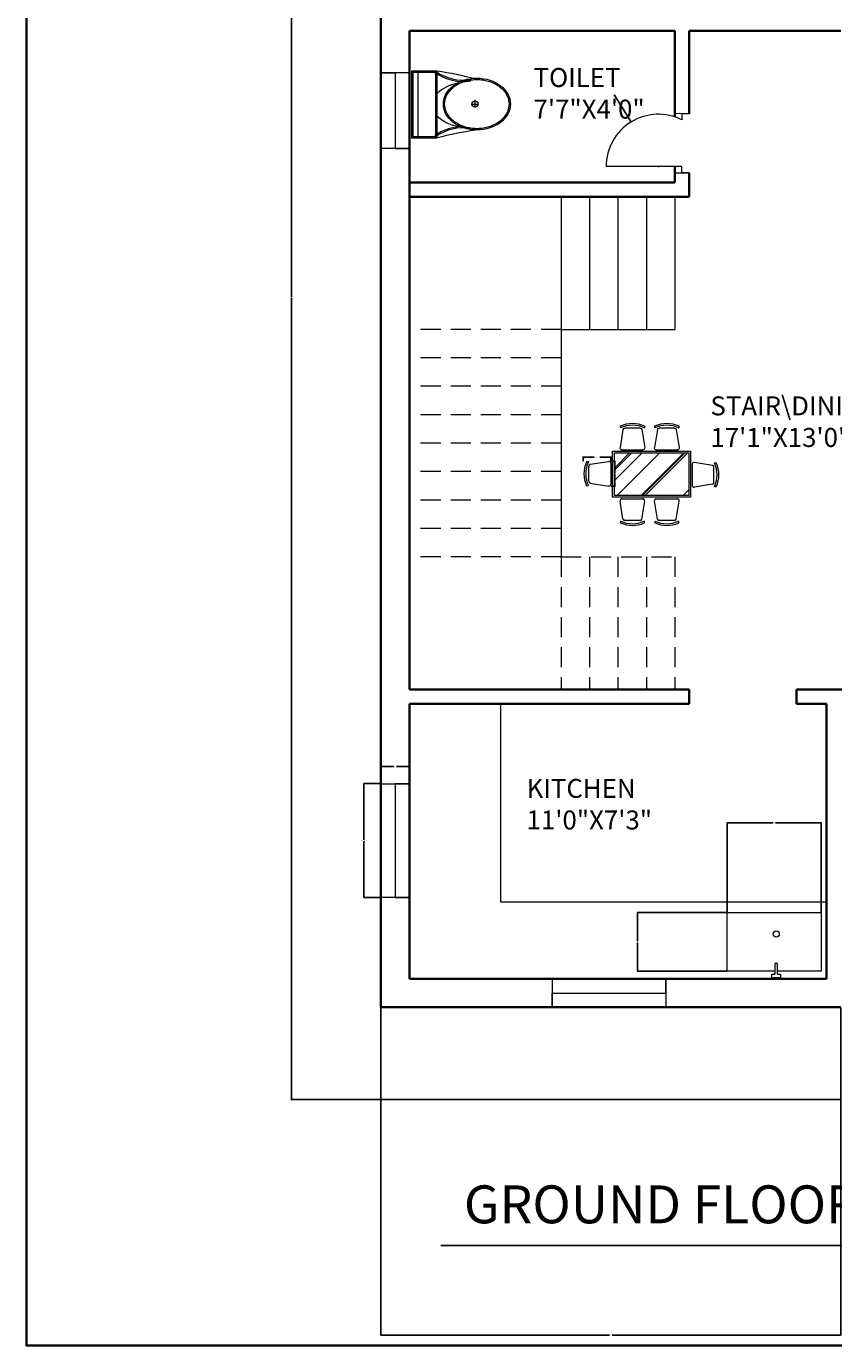
# Model space of a CAD drawing. Units: inches. Extents: x 1832 to 2989, y 1644 to 2902.
# Tile 1 of 8: x 1832 to 2087, y 1644 to 2061. Entities that reach past the tile are written whole.
import ezdxf

# ---------------------------------------------------------------- set-up
doc = ezdxf.new("R2010")
doc.units = ezdxf.units.IN
doc.linetypes.add('DASHED2', pattern=[9.525, 6.35, -3.175])
for name, color, linetype, lineweight in [('A-ANNO-DIMS', 2, 'Continuous', 18), ('A-ANNO-TEXT', 7, 'Continuous', 25), ('A-ANNO-TTLB', 7, 'Continuous', 35), ('A-AREA-IDEN', 7, 'Continuous', 18), ('A-DOOR', 3, 'Continuous', 18), ('A-FLOR-CASE', 8, 'Continuous', 18), ('A-FLOR-FIXT', 9, 'Continuous', 18), ('A-FLOR-STRS', 7, 'Continuous', 18), ('A-FLOR-STRS-OVHD', 254, 'DASHED2', 13), ('A-FURN', 8, 'Continuous', 18), ('A-FURN-PATT', 252, 'Continuous', 13), ('A-GLAZ', 4, 'Continuous', 18), ('A-WALL', 7, 'Continuous', 35)]:
    doc.layers.add(name, color=color, linetype=linetype, lineweight=lineweight)
doc.styles.get("Standard").update_dxf_attribs({"font": 'arial.ttf'})
doc.dimstyles.get("Standard").update_dxf_attribs({"dimtxt": 0.18, "dimasz": 0.18, "dimexe": 0.18, "dimexo": 0.0625, "dimgap": 0.09, "dimtad": 0, "dimtih": 1, "dimtoh": 1, "dimdec": 4, "dimzin": 0, "dimdsep": 46, "dimtxsty": 'Standard', "dimcen": 0.09, "dimadec": 0, "dimazin": 0, "dimtfac": 1, "dimtdec": 4, "dimtofl": 0, "dimtmove": 0, "dimatfit": 3, "dimfxl": 1, "dimtolj": 1, "dimtzin": 0, "dimarcsym": 0})

# ---------------------------------------------------------------- blocks, each defined once
blk = doc.blocks.new('A$C31115884')
for p, q in [((258, 466), (258, 523)), ((283, 498), (223, 498)), ((0, 200), (0, 0)), ((520, 200), (0, 200)), ((10, 190), (10, 10)), ((510, 190), (10, 190)), ((510, 10), (510, 190)), ((520, 0), (520, 200)), ((510, 54), (0, 54)), ((10, 10), (510, 10)), ((0, 0), (520, 0))]:
    blk.add_line(p, q)
blk.add_circle((256, 496), 23.6)
for centre, radius, start, end in [((2778, -205), 2807, 165.4549, 171.7133), ((-295, 403), 365, 324.2091, 9.3499), ((-295, 403), 375, 324.2091, 9.3499), ((139, 406), 293, 315.8436, 2.6563), ((806, 403), 365, 170.6501, 215.7909), ((3237, 905), 2807, 188.2867, 194.5451), ((384, 406), 293, 190.2774, 224.1564), ((806, 403), 375, 179.2036, 215.7909)]:
    blk.add_arc(centre, radius, start, end)
blk.add_ellipse((256, 510), major_axis=(0, -261), ratio=0.772727)
blk.add_open_spline([(256, 259), (263, 259), (270, 260), (288, 262), (299, 265), (320, 273), (330, 278), (350, 291), (360, 299), (378, 316), (386, 326), (402, 347), (409, 358), (421, 383), (427, 395), (436, 422), (440, 436), (445, 465), (447, 480), (448, 509), (448, 524), (445, 553), (443, 568), (436, 596), (432, 610), (422, 636), (416, 649), (402, 672), (395, 683), (379, 703), (370, 712), (351, 728), (341, 735), (321, 746), (310, 751), (289, 757), (278, 759), (256, 761), (245, 761), (223, 757), (212, 754), (191, 746), (181, 741), (161, 728), (151, 720), (133, 703), (125, 693), (110, 672), (103, 660), (90, 636), (85, 623), (76, 596), (72, 582), (67, 553), (66, 538), (64, 509), (65, 494), (68, 465), (70, 450), (77, 422), (81, 408), (91, 382), (97, 370), (111, 346), (118, 335), (135, 316), (144, 307), (162, 291), (172, 284), (193, 273), (203, 269), (225, 262), (236, 260), (250, 259), (253, 259), (256, 259)], degree=3, knots=[0, 0, 0, 0, 0.110105, 0.110105, 0.285049, 0.285049, 0.459994, 0.459994, 0.634938, 0.634938, 0.809882, 0.809882, 0.984827, 0.984827, 1.159771, 1.159771, 1.334715, 1.334715, 1.50966, 1.50966, 1.684604, 1.684604, 1.859549, 1.859549, 2.034493, 2.034493, 2.209437, 2.209437, 2.384382, 2.384382, 2.559326, 2.559326, 2.73427, 2.73427, 2.909215, 2.909215, 3.084159, 3.084159, 3.259103, 3.259103, 3.434048, 3.434048, 3.608992, 3.608992, 3.783936, 3.783936, 3.958881, 3.958881, 4.133825, 4.133825, 4.30877, 4.30877, 4.483714, 4.483714, 4.658658, 4.658658, 4.833603, 4.833603, 5.008547, 5.008547, 5.183491, 5.183491, 5.358436, 5.358436, 5.53338, 5.53338, 5.708324, 5.708324, 5.883269, 5.883269, 6.058213, 6.058213, 6.233158, 6.233158, 6.283185, 6.283185, 6.283185, 6.283185])
blk = doc.blocks.new('CHAIR-DINING')
for p, q in [((0.57, 8.47), (7.25, 8.47)), ((0.93, 2.02), (0, 7.73)), ((6.9, 2.02), (7.83, 7.73)), ((0.12, 1.4), (0.14, 0.86)), ((6.32, 1.56), (1.51, 1.56)), ((7.71, 0.84), (7.69, 1.42))]:
    blk.add_line(p, q)
for centre, radius, start, end in [((0.57, 7.92), 0.547, 90, 192.3792), ((7.25, 7.92), 0.547, 346.3053, 90), ((3.9, 9.34), 8.78, 244.6873, 295.6189), ((3.95, 8.89), 8.89, 244.649, 295.0455), ((1.51, 2.11), 0.547, 193.6947, 269.5544), ((6.32, 2.11), 0.547, 270.4456, 346.3053)]:
    blk.add_arc(centre, radius, start, end)
blk = doc.blocks.new('WIN-PLAN-24IN')
for p, q in [((0, 9), (0, 0)), ((24, 4.5), (24, 9)), ((24, 9), (24, 0)), ((0, 0), (0, 4.5)), ((0, 4.5), (24, 4.5))]:
    blk.add_line(p, q)
blk = doc.blocks.new('WIN-PLAN-36IN')
for p, q in [((0, 9), (0, 0)), ((36, 4.5), (36, 9)), ((36, 9), (36, 0)), ((0, 0), (0, 4.5)), ((0, 4.5), (36, 4.5))]:
    blk.add_line(p, q)
blk = doc.blocks.new('WIN-PLAN-36IN-2')
for p, q in [((0, 36), (9, 36)), ((9, 36), (4.5, 36)), ((4.5, 36), (4.5, 0)), ((9, 0), (0, 0)), ((4.5, 0), (9, 0))]:
    blk.add_line(p, q)
blk = doc.blocks.new('DOOR-PLAN-WC')
for p, q in [((21.75, 18.87), (26.25, 18.72)), ((26.25, 18.72), (24, 18.8)), ((24, 18.8), (24, 16.8)), ((24, 2), (0, 2)), ((21.75, 0), (26.25, 0)), ((24, 0), (24, 2)), ((26.25, 0), (24, 0))]:
    blk.add_line(p, q)
blk.add_arc((16.56, 2), 16.56, 63.308, 180)
blk = doc.blocks.new('*D29')
at = {"layer": 'A-ANNO-DIMS', "color": 0, "lineweight": -2, "transparency": 16777216}
for p, q in [((2007.84, 1923.49), (2007.84, 1924.92)), ((2008.02, 1924.74), (2011.33, 1924.74)), ((2016.41, 1924.74), (2013.1, 1924.74)), ((2016.59, 1923.49), (2016.59, 1924.92))]:
    blk.add_line(p, q, dxfattribs=at)
at = {"layer": 'A-ANNO-DIMS', "color": 0, "transparency": 16777216}
for points in [[(2008.02, 1924.77), (2008.02, 1924.71), (2007.84, 1924.74)], [(2016.41, 1924.77), (2016.41, 1924.71), (2016.59, 1924.74)]]:
    blk.add_solid(points, dxfattribs=at)
at = {"layer": 'Defpoints', "color": 0, "transparency": 16777216}
for p in [(2016.59, 1924.74), (2007.84, 1923.42), (2016.59, 1923.42)]:
    blk.add_point(p, dxfattribs=at)
at = {"layer": 'A-ANNO-DIMS', "color": 0, "transparency": 16777216, "insert": (2012.21, 1924.74), "char_height": 0.18, "attachment_point": 5}
blk.add_mtext('\\A1;CHAIR 9 TYP.', dxfattribs=at)
blk = doc.blocks.new('*D30')
at = {"layer": 'A-ANNO-DIMS', "color": 0, "lineweight": -2, "transparency": 16777216}
for p, q in [((2016.65, 1923.42), (2018.08, 1923.42)), ((2017.9, 1923.24), (2017.9, 1919.69)), ((2017.9, 1915.78), (2017.9, 1919.33)), ((2016.65, 1915.6), (2018.08, 1915.6))]:
    blk.add_line(p, q, dxfattribs=at)
at = {"layer": 'A-ANNO-DIMS', "color": 0, "transparency": 16777216}
for points in [[(2017.87, 1923.24), (2017.93, 1923.24), (2017.9, 1923.42)], [(2017.87, 1915.78), (2017.93, 1915.78), (2017.9, 1915.6)]]:
    blk.add_solid(points, dxfattribs=at)
at = {"layer": 'Defpoints', "color": 0, "transparency": 16777216}
for p in [(2016.59, 1923.42), (2016.59, 1915.6), (2017.9, 1915.6)]:
    blk.add_point(p, dxfattribs=at)
at = {"layer": 'A-ANNO-DIMS', "color": 0, "transparency": 16777216, "insert": (2017.9, 1919.51), "char_height": 0.18, "attachment_point": 5}
blk.add_mtext('\\A1;8 TYP.', dxfattribs=at)
blk = doc.blocks.new('*D57')
at = {"layer": 'A-ANNO-DIMS', "color": 0, "lineweight": -2, "transparency": 16777216}
for p, q in [((1943.83, 1821.42), (1938.31, 1821.42)), ((1938.49, 1821.24), (1938.49, 1803.6)), ((1938.49, 1785.6), (1938.49, 1803.23)), ((1943.83, 1785.42), (1938.31, 1785.42))]:
    blk.add_line(p, q, dxfattribs=at)
at = {"layer": 'A-ANNO-DIMS', "color": 0, "transparency": 16777216}
for points in [[(1938.46, 1821.24), (1938.52, 1821.24), (1938.49, 1821.42)], [(1938.46, 1785.6), (1938.52, 1785.6), (1938.49, 1785.42)]]:
    blk.add_solid(points, dxfattribs=at)
at = {"layer": 'Defpoints', "color": 0, "transparency": 16777216}
for p in [(1938.49, 1821.42), (1943.89, 1821.42), (1943.89, 1785.42)]:
    blk.add_point(p, dxfattribs=at)
at = {"layer": 'A-ANNO-DIMS', "color": 0, "transparency": 16777216, "insert": (1938.49, 1803.42), "char_height": 0.18, "attachment_point": 5}
blk.add_mtext('\\A1;WINDOW 36 TYP.', dxfattribs=at)
blk = doc.blocks.new('*D58')
at = {"layer": 'A-ANNO-DIMS', "color": 0, "lineweight": -2, "transparency": 16777216}
for p, q in [((1943.89, 1821.48), (1943.89, 1827)), ((1944.07, 1826.82), (1947.93, 1826.82)), ((1952.71, 1826.82), (1948.85, 1826.82)), ((1952.89, 1821.48), (1952.89, 1827))]:
    blk.add_line(p, q, dxfattribs=at)
at = {"layer": 'A-ANNO-DIMS', "color": 0, "transparency": 16777216}
for points in [[(1944.07, 1826.85), (1944.07, 1826.79), (1943.89, 1826.82)], [(1952.71, 1826.85), (1952.71, 1826.79), (1952.89, 1826.82)]]:
    blk.add_solid(points, dxfattribs=at)
at = {"layer": 'Defpoints', "color": 0, "transparency": 16777216}
for p in [(1952.89, 1826.82), (1943.89, 1821.42), (1952.89, 1821.42)]:
    blk.add_point(p, dxfattribs=at)
at = {"layer": 'A-ANNO-DIMS', "color": 0, "transparency": 16777216, "insert": (1948.39, 1826.82), "char_height": 0.18, "attachment_point": 5}
blk.add_mtext('\\A1;9 TYP.', dxfattribs=at)
blk = doc.blocks.new('*D72')
at = {"layer": 'A-ANNO-DIMS', "color": 0, "lineweight": -2, "transparency": 16777216}
for p, q in [((1943.83, 2229.17), (1915.41, 2229.17)), ((1915.59, 2228.99), (1915.59, 1975.53)), ((1915.59, 1721.7), (1915.59, 1975.17)), ((2089.33, 1721.52), (1915.41, 1721.52))]:
    blk.add_line(p, q, dxfattribs=at)
at = {"layer": 'A-ANNO-DIMS', "color": 0, "transparency": 16777216}
for points in [[(1915.56, 2228.99), (1915.62, 2228.99), (1915.59, 2229.17)], [(1915.56, 1721.7), (1915.62, 1721.7), (1915.59, 1721.52)]]:
    blk.add_solid(points, dxfattribs=at)
at = {"layer": 'Defpoints', "color": 0, "transparency": 16777216}
for p in [(1915.59, 2229.17), (1943.89, 2229.17), (2089.39, 1721.52)]:
    blk.add_point(p, dxfattribs=at)
at = {"layer": 'A-ANNO-DIMS', "color": 0, "transparency": 16777216, "insert": (1915.59, 1975.35), "char_height": 0.18, "attachment_point": 5}
blk.add_mtext('\\A1;507.6', dxfattribs=at)
blk = doc.blocks.new('*D75')
at = {"layer": 'A-ANNO-DIMS', "color": 0, "lineweight": -2, "transparency": 16777216}
for p, q in [((1943.89, 1750.61), (1943.89, 1646.75)), ((2089.39, 1750.61), (2089.39, 1646.75)), ((1944.07, 1646.93), (2016.25, 1646.93)), ((2089.21, 1646.93), (2017.03, 1646.93))]:
    blk.add_line(p, q, dxfattribs=at)
at = {"layer": 'A-ANNO-DIMS', "color": 0, "transparency": 16777216}
for points in [[(1944.07, 1646.96), (1944.07, 1646.9), (1943.89, 1646.93)], [(2089.21, 1646.96), (2089.21, 1646.9), (2089.39, 1646.93)]]:
    blk.add_solid(points, dxfattribs=at)
at = {"layer": 'Defpoints', "color": 0, "transparency": 16777216}
for p in [(1943.89, 1750.67), (2089.39, 1750.67), (2089.39, 1646.93)]:
    blk.add_point(p, dxfattribs=at)
at = {"layer": 'A-ANNO-DIMS', "color": 0, "transparency": 16777216, "insert": (2016.64, 1646.93), "char_height": 0.18, "attachment_point": 5}
blk.add_mtext('\\A1;145.5', dxfattribs=at)
blk = doc.blocks.new('*D79')
at = {"layer": 'A-ANNO-DIMS', "color": 0, "lineweight": -2, "transparency": 16777216}
for p, q in [((2053.41, 1780.75), (2053.41, 1809.16)), ((2053.59, 1808.98), (2067.86, 1808.98)), ((2083.06, 1808.98), (2068.79, 1808.98)), ((2083.24, 1780.75), (2083.24, 1809.16))]:
    blk.add_line(p, q, dxfattribs=at)
at = {"layer": 'A-ANNO-DIMS', "color": 0, "transparency": 16777216}
for points in [[(2053.59, 1809.01), (2053.59, 1808.95), (2053.41, 1808.98)], [(2083.06, 1809.01), (2083.06, 1808.95), (2083.24, 1808.98)]]:
    blk.add_solid(points, dxfattribs=at)
at = {"layer": 'Defpoints', "color": 0, "transparency": 16777216}
for p in [(2083.24, 1808.98), (2053.41, 1780.68), (2083.24, 1780.68)]:
    blk.add_point(p, dxfattribs=at)
at = {"layer": 'A-ANNO-DIMS', "color": 0, "transparency": 16777216, "insert": (2068.33, 1808.98), "char_height": 0.18, "attachment_point": 5}
blk.add_mtext('\\A1;29.833', dxfattribs=at)
blk = doc.blocks.new('*D80')
at = {"layer": 'A-ANNO-DIMS', "color": 0, "lineweight": -2, "transparency": 16777216}
for p, q in [((2053.35, 1780.68), (2024.93, 1780.68)), ((2025.11, 1780.5), (2025.11, 1771.56)), ((2025.11, 1762.26), (2025.11, 1771.2)), ((2053.35, 1762.08), (2024.93, 1762.08))]:
    blk.add_line(p, q, dxfattribs=at)
at = {"layer": 'A-ANNO-DIMS', "color": 0, "transparency": 16777216}
for points in [[(2025.08, 1780.5), (2025.14, 1780.5), (2025.11, 1780.68)], [(2025.08, 1762.26), (2025.14, 1762.26), (2025.11, 1762.08)]]:
    blk.add_solid(points, dxfattribs=at)
at = {"layer": 'Defpoints', "color": 0, "transparency": 16777216}
for p in [(2025.11, 1780.68), (2053.41, 1780.68), (2053.41, 1762.08)]:
    blk.add_point(p, dxfattribs=at)
at = {"layer": 'A-ANNO-DIMS', "color": 0, "transparency": 16777216, "insert": (2025.11, 1771.38), "char_height": 0.18, "attachment_point": 5}
blk.add_mtext('\\A1;18.61', dxfattribs=at)
blk = doc.blocks.new('*D127')
at = {"layer": 'A-ANNO-DIMS', "color": 0, "lineweight": -2, "transparency": 16777216}
for p, q in [((2017.62, 2039.25), (2017.8, 2039.25)), ((2017.8, 2039.25), (2022.92, 2030.95)), ((2031.61, 2016.7), (2031.79, 2016.7)), ((2031.7, 2016.61), (2031.7, 2016.79))]:
    blk.add_line(p, q, dxfattribs=at)
at = {"layer": 'A-ANNO-DIMS', "color": 0, "transparency": 16777216}
blk.add_solid([(2022.94, 2030.96), (2022.89, 2030.93), (2023.01, 2030.8)], dxfattribs=at)
at = {"layer": 'Defpoints', "color": 0, "transparency": 16777216}
for p in [(2023.01, 2030.8), (2031.7, 2016.7)]:
    blk.add_point(p, dxfattribs=at)
at = {"layer": 'A-ANNO-DIMS', "color": 0, "transparency": 16777216, "insert": (2017.14, 2039.25), "char_height": 0.18, "attachment_point": 5}
blk.add_mtext('\\A1;R16.56', dxfattribs=at)

msp = doc.modelspace()

# ---------------------------------------------------------------- hatches: boundary and pattern name
at = {"layer": 'A-FURN-PATT'}
h = msp.add_hatch(dxfattribs=at)
h.set_pattern_fill('AR-RROOF', color=256, scale=0.368444, angle=45, style=0)
h.set_pattern_definition([(45, (1517.465, 2118.481), (7.94093, 21.1758), [140.3771, -18.717, 46.7924, -9.3585]), (45, (1522.958, 2130.591), (-15.41863, 2.18375), [28.0754, -3.0883, 56.1508, -7.01885]), (45, (1515.149, 2127.4145), (29.977, 38.84437), [74.8678, -13.10186, 37.4339, -9.3585])])
h.paths.add_polyline_path([(2017.7478, 1926.1046), (2017.7478, 1912.603), (2041.3439, 1912.603), (2041.3439, 1926.1046)])

# ---------------------------------------------------------------- linework, layer by layer
at = {"layer": 'A-ANNO-TEXT'}
msp.add_line((1962.8459, 1675.2337), (2280.5653, 1675.2337), dxfattribs=at)
at = {"layer": 'A-ANNO-TTLB'}
msp.add_lwpolyline([(1831.6677, 2901.9044), (2988.9144, 2901.9044), (2988.9144, 1643.5851), (1831.6677, 1643.5851)], close=True, dxfattribs=at)
at = {"layer": 'A-FLOR-CASE'}
for p, q in [((1981.754, 1846.6726), (1981.754, 1784.0547)), ((1981.754, 1784.0547), (2084.8904, 1784.0547))]:
    msp.add_line(p, q, dxfattribs=at)
at = {"layer": 'A-FLOR-FIXT'}
for points in [[(2068.5195, 1762.076), (2053.4086, 1762.076), (2053.4086, 1780.6849), (2083.2418, 1780.6849), (2083.2418, 1762.076), (2069.3589, 1762.076)], [(2069.3589, 1761.1417), (2069.3589, 1764.4617), (2068.5195, 1764.4617), (2068.5195, 1761.1417)], [(2069.3589, 1761.1417), (2070.335, 1761.1417), (2070.335, 1759.9628), (2067.6253, 1759.9628), (2067.6253, 1761.1417), (2068.5195, 1761.1417)]]:
    msp.add_lwpolyline(points, dxfattribs=at)
msp.add_circle((2068.9811, 1773.831), 0.9741, dxfattribs=at)
at = {"layer": 'A-FLOR-STRS'}
for p, q in [((1952.8904, 2007.1726), (2000.8904, 2007.1726)), ((2000.8904, 2007.1726), (2000.8904, 1959.1726)), ((2000.8904, 2007.1726), (2000.8904, 1965.1726)), ((2009.8904, 2007.1726), (2009.8904, 1965.1726)), ((2018.8904, 2007.1726), (2018.8904, 1965.1726)), ((2027.8904, 2007.1726), (2027.8904, 1965.1726)), ((2036.8904, 2007.1726), (2036.8904, 1965.1726)), ((2000.8904, 1965.1726), (2036.8904, 1965.1726)), ((2000.8904, 1959.1726), (2000.8904, 1893.1726))]:
    msp.add_line(p, q, dxfattribs=at)
at = {"layer": 'A-FLOR-STRS-OVHD'}
for p, q in [((2000.8904, 1965.1726), (1952.8904, 1965.1726)), ((2000.8904, 1956.1726), (1952.8904, 1956.1726)), ((2000.8904, 1947.1726), (1952.8904, 1947.1726)), ((2000.8904, 1938.1726), (1952.8904, 1938.1726)), ((2000.8904, 1929.1726), (1952.8904, 1929.1726)), ((2000.8904, 1920.1726), (1952.8904, 1920.1726)), ((2000.8904, 1911.1726), (1952.8904, 1911.1726)), ((2000.8904, 1902.1726), (1952.8904, 1902.1726)), ((2000.8904, 1893.1726), (1952.8904, 1893.1726)), ((2000.8904, 1893.1726), (2000.8904, 1851.1726)), ((2000.8904, 1893.1726), (2036.8904, 1893.1726)), ((2009.8904, 1893.1726), (2009.8904, 1851.1726)), ((2018.8904, 1893.1726), (2018.8904, 1851.1726)), ((2027.8904, 1893.1726), (2027.8904, 1851.1726)), ((2036.8904, 1893.1726), (2036.8904, 1851.1726))]:
    msp.add_line(p, q, dxfattribs=at)
at = {"layer": 'A-FURN'}
for p, q in [((2042.359, 1922.4877), (2042.359, 1915.8087)), ((2048.803, 1922.1324), (2043.0983, 1923.0614)), ((2049.2644, 1916.7417), (2049.2644, 1921.5547)), ((2049.4269, 1922.9372), (2049.9717, 1922.9171)), ((2048.803, 1916.1639), (2043.0983, 1915.2349)), ((2049.9918, 1915.3468), (2049.4067, 1915.367))]:
    msp.add_line(p, q, dxfattribs=at)
for points in [[(2017.1952, 1926.6572), (2041.8965, 1926.6572), (2041.8965, 1912.0503), (2017.1952, 1912.0503)], [(2017.7478, 1926.1046), (2041.3439, 1926.1046), (2041.3439, 1912.603), (2017.7478, 1912.603)]]:
    msp.add_lwpolyline(points, close=True, dxfattribs=at)
for centre, radius, start, end in [((2042.9062, 1922.4877), 0.5471, 77.620777, 180), ((2048.7173, 1921.5504), 0.5471, 0.445647, 76.305274), ((2041.4901, 1919.1632), 8.7797, 334.381056, 25.312705), ((2041.9373, 1919.1105), 8.8905, 334.954464, 25.350959), ((2048.6266, 1916.7779), 0.6388, 286.031111, 356.752573), ((2042.9787, 1915.8439), 0.6206, 183.254478, 281.116612)]:
    msp.add_arc(centre, radius, start, end, dxfattribs=at)
at = {"layer": 'A-WALL'}
for p, q in [((1943.8904, 2229.1726), (1943.8904, 1750.6726)), ((1943.8904, 2229.1726), (1943.8904, 1750.6726)), ((1943.8904, 2229.1726), (1943.8904, 1750.6726)), ((1952.8904, 2059.6726), (2036.8904, 2059.6726)), ((1952.8904, 2059.6726), (1952.8904, 1851.1726)), ((2036.8904, 2059.6726), (2036.8904, 2032.4253)), ((2041.3904, 2059.6726), (2041.3904, 2033.4226)), ((2041.3904, 2059.6726), (2089.3904, 2059.6726)), ((2036.8904, 2016.6983), (2036.8904, 2011.6726)), ((2041.3904, 2014.6983), (2041.3904, 2007.1726)), ((1952.8904, 2011.6726), (2036.8904, 2011.6726)), ((1952.8904, 2007.1726), (2041.3904, 2007.1726)), ((1952.8904, 1851.1726), (2010.6177, 1851.1726)), ((2010.6177, 1851.1726), (2041.3904, 1851.1726)), ((2041.3904, 1851.1726), (2041.3904, 1846.6726)), ((2075.4242, 1851.1726), (2075.4242, 1846.6726)), ((2075.4242, 1851.1726), (2096.7965, 1851.1726)), ((1952.8904, 1846.6726), (2010.6177, 1846.6726)), ((1952.8904, 1846.6726), (1952.8904, 1759.6726)), ((2041.3904, 1846.6726), (2010.6177, 1846.6726)), ((2041.3904, 1849.0845), (2041.3904, 1846.6726)), ((2075.4242, 1846.6726), (2084.8904, 1846.6726)), ((2084.8904, 1846.6726), (2084.8904, 1759.6726)), ((1952.8904, 1759.6726), (2084.8904, 1759.6726)), ((1952.8904, 1750.6726), (1943.8904, 1750.6726)), ((1952.8904, 1750.6726), (2089.3904, 1750.6726))]:
    msp.add_line(p, q, dxfattribs=at)

# ---------------------------------------------------------------- block references
at = {"layer": 'A-DOOR'}
msp.add_blockref('DOOR-PLAN-WC', (2015.1404, 2014.6983), dxfattribs=at)
at = {"layer": 'A-FLOR-FIXT', "xscale": 0.0406268506401408, "yscale": 0.0406268506401408, "zscale": 0.0406268506401408, "rotation": 269.9999999999998}
msp.add_blockref('A$C31115884', (1953.5142, 2046.8898), dxfattribs=at)
at = {"layer": 'A-FURN', "extrusion": (0, 0, -1), "zscale": -1, "rotation": 180}
for p in [(-2019.5519, 1935.4903), (-2030.4428, 1935.4903)]:
    msp.add_blockref('CHAIR-DINING', p, dxfattribs=at)
at = {"layer": 'A-FURN', "rotation": 269.9999999432575}
msp.add_blockref('CHAIR-DINING', (2008.1214, 1923.4234), dxfattribs=at)
at = {"layer": 'A-FURN'}
for p in [(2019.5519, 1903.1223), (2030.4428, 1903.1223)]:
    msp.add_blockref('CHAIR-DINING', p, dxfattribs=at)
at = {"layer": 'A-GLAZ', "rotation": 270.0000000000013}
msp.add_blockref('WIN-PLAN-24IN', (1943.8904, 2046.3857), dxfattribs=at)
at = {"layer": 'A-GLAZ'}
for name, p in [('WIN-PLAN-36IN-2', (1943.8904, 1785.4153)), ('WIN-PLAN-36IN', (1998.0413, 1750.6726))]:
    msp.add_blockref(name, p, dxfattribs=at)

# ---------------------------------------------------------------- texts
at = {"layer": 'A-ANNO-TEXT', "insert": (1970.1351, 1694.2857), "char_height": 12, "attachment_point": 1}
msp.add_mtext_dynamic_manual_height_columns('GROUND FLOOR EAST FACING PLAN', width=528.005294, gutter_width=12.5, heights=[0], dxfattribs=at)
at = {"layer": 'A-AREA-IDEN', "char_height": 6, "attachment_point": 1}
for s, width, insert in [('TOILET\\P7\'7"X4\'0"', 102.121913, (1992.1671, 2047.8855)), ('STAIR\\\\DINING\\P17\'1"X13\'0"', 222.625783, (2048.147, 1943.978)), ('KITCHEN\\P11\'0"X7\'3"', 205.6642, (1989.9623, 1822.9307))]:
    msp.add_mtext_dynamic_manual_height_columns(s, width=width, gutter_width=12.5, heights=[0], dxfattribs=dict(at, insert=insert))

# ---------------------------------------------------------------- dimensions: what is measured, and where the dimension line sits
at = {"layer": 'A-ANNO-DIMS'}
for base, p1, p2, override, picture, middle in [((1915.5904, 2229.1726), (2089.3904, 1721.5243), (1943.8904, 2229.1726), {"dimdec": 1, "dimlfac": 1, "dimrnd": 0, "dimzin": 0, "dimdsep": 46, "dimlunit": 2}, '*D72', (1915.5904, 1975.3484)), ((2025.1086, 1780.6849), (2053.4086, 1762.076), (2053.4086, 1780.6849), {"dimdec": 2, "dimlfac": 1, "dimrnd": 0, "dimzin": 0, "dimdsep": 46, "dimlunit": 2}, '*D80', (2025.1086, 1771.3805))]:
    dim = msp.add_linear_dim(base=base, p1=p1, p2=p2, angle=90, dimstyle='Standard', override=override, dxfattribs=at)
    dim.commit()
    dim.dimension.update_dxf_attribs({"geometry": picture, "text_midpoint": middle})
dim = msp.add_radius_dim(center=(2031.7013, 2016.6983), mpoint=(2023.0103, 2030.7955), dimstyle='Standard', override={"dimdec": 2, "dimlfac": 1, "dimrnd": 0, "dimzin": 0, "dimdsep": 46, "dimlunit": 2}, dxfattribs=at)
dim.commit()
dim.dimension.update_dxf_attribs({"geometry": '*D127', "text_midpoint": (2017.1359, 2039.2538), "dimtype": 164})
for base, p1, p2, angle, text, picture, middle in [((2016.5901, 1924.7366), (2007.8357, 1923.4234), (2016.5901, 1923.4234), 360, 'CHAIR <> TYP.', '*D29', (2012.2129, 1924.7366)), ((2017.9033, 1915.597), (2016.5901, 1923.4234), (2016.5901, 1915.597), 270, '<> TYP.', '*D30', (2017.9033, 1919.5102)), ((1938.4904, 1821.4153), (1943.8904, 1785.4153), (1943.8904, 1821.4153), 90, 'WINDOW <> TYP.', '*D57', (1938.4904, 1803.4153))]:
    dim = msp.add_linear_dim(base=base, p1=p1, p2=p2, angle=angle, text=text, dimstyle='Standard', override={"dimdec": 0, "dimlfac": 1, "dimrnd": 0, "dimzin": 0, "dimdsep": 46, "dimlunit": 2}, dxfattribs=at)
    dim.commit()
    dim.dimension.update_dxf_attribs({"geometry": picture, "text_midpoint": middle})
dim = msp.add_linear_dim(base=(1952.8904, 1826.8153), p1=(1943.8904, 1821.4153), p2=(1952.8904, 1821.4153), text='<> TYP.', dimstyle='Standard', override={"dimdec": 0, "dimlfac": 1, "dimrnd": 0, "dimzin": 0, "dimdsep": 46, "dimlunit": 2}, dxfattribs=at)
dim.commit()
dim.dimension.update_dxf_attribs({"geometry": '*D58', "text_midpoint": (1948.3904, 1826.8153)})
for base, p1, p2, override, picture, middle in [((2083.2418, 1808.9849), (2053.4086, 1780.6849), (2083.2418, 1780.6849), {"dimdec": 3, "dimlfac": 1, "dimrnd": 0, "dimzin": 0, "dimdsep": 46, "dimlunit": 2}, '*D79', (2068.3252, 1808.9849)), ((2089.3904, 1646.9337), (1943.8904, 1750.6726), (2089.3904, 1750.6726), {"dimdec": 1, "dimlfac": 1, "dimrnd": 0, "dimzin": 0, "dimdsep": 46, "dimlunit": 2}, '*D75', (2016.6404, 1646.9337))]:
    dim = msp.add_linear_dim(base=base, p1=p1, p2=p2, dimstyle='Standard', override=override, dxfattribs=at)
    dim.commit()
    dim.dimension.update_dxf_attribs({"geometry": picture, "text_midpoint": middle})

doc.saveas('drawing.dxf')
